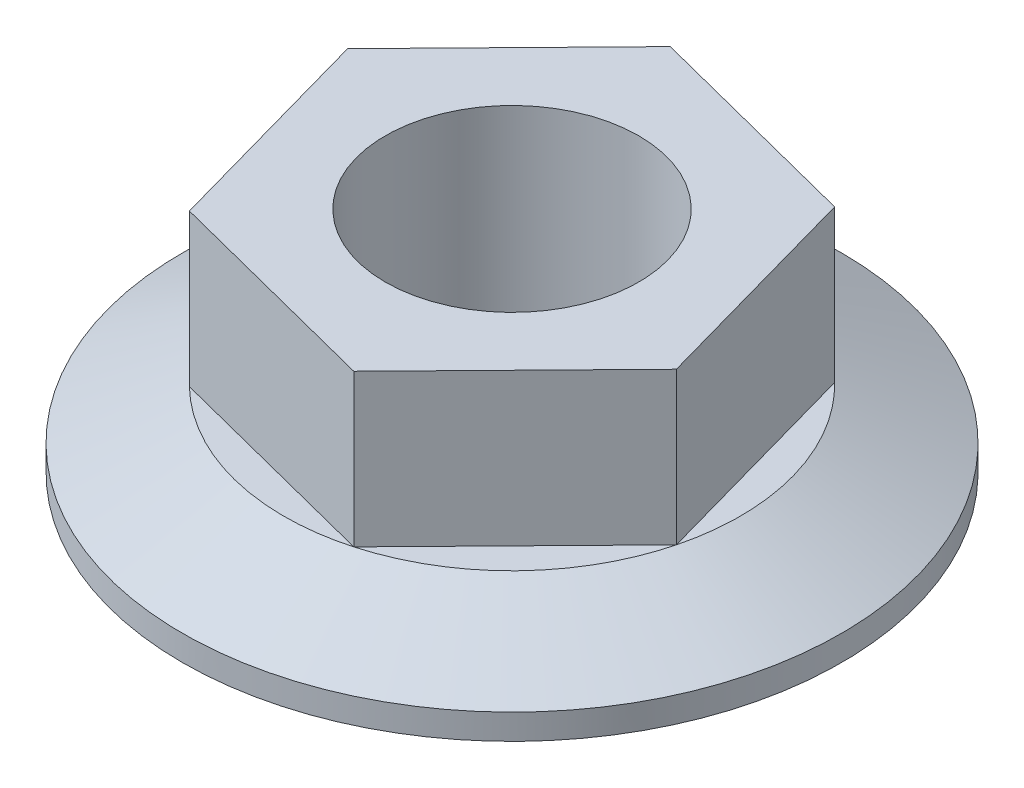
ISO-10303-21;
HEADER;
FILE_DESCRIPTION(('STEP AP214'),'2;1');
FILE_NAME('part.step','',(''),(''),'','','');
FILE_SCHEMA(('AUTOMOTIVE_DESIGN { 1 0 10303 214 1 1 1 1 }'));
ENDSEC;
DATA;
#1=APPLICATION_CONTEXT('core data for automotive mechanical design processes');
#2=APPLICATION_PROTOCOL_DEFINITION('international standard','automotive_design',2000,#1);
#3=PRODUCT_CONTEXT('',#1,'mechanical');
#4=PRODUCT('Part','Part','',(#3));
#5=PRODUCT_RELATED_PRODUCT_CATEGORY('part','',(#4));
#6=PRODUCT_DEFINITION_FORMATION('','',#4);
#7=PRODUCT_DEFINITION_CONTEXT('part definition',#1,'design');
#8=PRODUCT_DEFINITION('design','',#6,#7);
#9=PRODUCT_DEFINITION_SHAPE('','',#8);
#10=(LENGTH_UNIT() NAMED_UNIT(*) SI_UNIT(.MILLI.,.METRE.));
#11=(NAMED_UNIT(*) PLANE_ANGLE_UNIT() SI_UNIT($,.RADIAN.));
#12=(NAMED_UNIT(*) SI_UNIT($,.STERADIAN.) SOLID_ANGLE_UNIT());
#13=UNCERTAINTY_MEASURE_WITH_UNIT(LENGTH_MEASURE(1.E-05),#10,'distance_accuracy_value','');
#14=(GEOMETRIC_REPRESENTATION_CONTEXT(3) GLOBAL_UNCERTAINTY_ASSIGNED_CONTEXT((#13)) GLOBAL_UNIT_ASSIGNED_CONTEXT((#10,
#11,#12)) REPRESENTATION_CONTEXT('',''));
#15=CARTESIAN_POINT('',(0.,0.,0.));
#16=DIRECTION('',(0.,0.,1.));
#17=DIRECTION('',(1.,0.,0.));
#18=AXIS2_PLACEMENT_3D('',#15,#16,#17);
#19=CARTESIAN_POINT('',(0.,1.5,0.));
#20=DIRECTION('',(0.,1.,0.));
#21=DIRECTION('',(0.,0.,1.));
#22=AXIS2_PLACEMENT_3D('',#19,#20,#21);
#23=PLANE('',#22);
#24=CARTESIAN_POINT('',(-3.14677034971334,1.5,3.21680530436099));
#25=CARTESIAN_POINT('',(-2.93612740137397,1.5,3.42286222154896));
#26=CARTESIAN_POINT('',(-2.69997194565525,1.5,3.60002104058776));
#27=CARTESIAN_POINT('',(-2.58257022633489,1.5,3.68809332282499));
#28=CARTESIAN_POINT('',(-2.4587384571172,1.5,3.76889973327667));
#29=CARTESIAN_POINT('',(-2.33582790103386,1.5,3.84910500617602));
#30=CARTESIAN_POINT('',(-2.20697627303336,1.5,3.92163941869568));
#31=CARTESIAN_POINT('',(-2.07908320205732,1.5,3.9936342309657));
#32=CARTESIAN_POINT('',(-1.94576347772724,1.5,4.05758604206279));
#33=CARTESIAN_POINT('',(-1.81343554962159,1.5,4.12106210086509));
#34=CARTESIAN_POINT('',(-1.67621862449045,1.5,4.17615745906585));
#35=CARTESIAN_POINT('',(-1.54002248775998,1.5,4.23084295017093));
#36=CARTESIAN_POINT('',(-1.39949594576583,1.5,4.27684592869383));
#37=CARTESIAN_POINT('',(-1.26001481317743,1.5,4.32250668043339));
#38=CARTESIAN_POINT('',(-1.1167804105469,1.5,4.35922028746182));
#39=CARTESIAN_POINT('',(-0.974611561722385,1.5,4.3956607734873));
#40=CARTESIAN_POINT('',(-0.829282650158769,1.5,4.42292779571922));
#41=CARTESIAN_POINT('',(-0.685034873936298,1.5,4.44999197227462));
#42=CARTESIAN_POINT('',(-0.538233774148871,1.5,4.46769564813512));
#43=CARTESIAN_POINT('',(-0.392524761650793,1.5,4.4852676222617));
#44=CARTESIAN_POINT('',(-0.244880098486916,1.5,4.49333214189259));
#45=CARTESIAN_POINT('',(-0.0983337980726981,1.5,4.50133666769934));
#46=CARTESIAN_POINT('',(0.0495221913514423,1.5,4.49972749758958));
#47=CARTESIAN_POINT('',(0.196278245921577,1.5,4.49813029846792));
#48=CARTESIAN_POINT('',(0.343712419563647,1.5,4.48685432933115));
#49=CARTESIAN_POINT('',(0.49004979633479,1.5,4.47566224473323));
#50=CARTESIAN_POINT('',(0.63643081842759,1.5,4.45476776200012));
#51=CARTESIAN_POINT('',(0.781722878287567,1.5,4.43402871815004));
#52=CARTESIAN_POINT('',(0.926423922820389,1.5,4.40360519520382));
#53=CARTESIAN_POINT('',(1.07031840990569,1.5,4.37335125167627));
#54=CARTESIAN_POINT('',(1.21244993774848,1.5,4.33358571490789));
#55=B_SPLINE_CURVE_WITH_KNOTS('',2,(#24,#25,#26,#27,#28,#29,#30,#31,#32,#33,#34,#35,#36,#37,#38,
#39,#40,#41,#42,#43,#44,#45,#46,#47,#48,#49,#50,#51,#52,#53,#54),.UNSPECIFIED.,.F.,.F.,(3,2,2,2,
2,2,2,2,2,2,2,2,2,2,2,3),(0.,0.125,0.1875,0.25,0.3125,0.375,0.4375,0.5,0.5625,0.625,0.6875,0.75,
0.8125,0.875,0.9375,1.),.UNSPECIFIED.);
#56=CARTESIAN_POINT('',(-3.14677034971334,1.5,3.21680530436099));
#57=VERTEX_POINT('',#56);
#58=CARTESIAN_POINT('',(1.21244944410103,1.5,4.33358395085455));
#59=VERTEX_POINT('',#58);
#60=EDGE_CURVE('E65',#57,#59,#55,.T.);
#61=ORIENTED_EDGE('',*,*,#60,.T.);
#62=DIRECTION('',(-0.96871561943596,0.,-0.248173424565978));
#63=VECTOR('',#62,1.);
#64=CARTESIAN_POINT('',(-0.967160205982432,1.5,3.77519550963444));
#65=LINE('',#64,#63);
#66=EDGE_CURVE('E12',#59,#57,#65,.T.);
#67=ORIENTED_EDGE('',*,*,#66,.T.);
#68=EDGE_LOOP('',(#61,#67));
#69=FACE_BOUND('',#68,.T.);
#70=ADVANCED_FACE('F44',(#69),#23,.T.);
#71=CARTESIAN_POINT('',(1.21244993774848,1.5,4.33358571490789));
#72=CARTESIAN_POINT('',(1.49622193684302,1.5,4.25419202910785));
#73=CARTESIAN_POINT('',(1.76772370250781,1.5,4.13825481472469));
#74=CARTESIAN_POINT('',(1.90269739596185,1.5,4.08061808445978));
#75=CARTESIAN_POINT('',(2.03459368481606,1.5,4.01377983174297));
#76=CARTESIAN_POINT('',(2.1655087667138,1.5,3.94743880422554));
#77=CARTESIAN_POINT('',(2.29275122460852,1.5,3.87211722731326));
#78=CARTESIAN_POINT('',(2.41904709647025,1.5,3.79735598500837));
#79=CARTESIAN_POINT('',(2.54109085166662,1.5,3.71387362245623));
#80=CARTESIAN_POINT('',(2.66222669517993,1.5,3.63101230448085));
#81=CARTESIAN_POINT('',(2.7785491375814,1.5,3.53972664058196));
#82=CARTESIAN_POINT('',(2.89400623046664,1.5,3.44912007182123));
#83=CARTESIAN_POINT('',(3.00410924951721,1.5,3.35042200580243));
#84=CARTESIAN_POINT('',(3.11339318677755,1.5,3.25245817749394));
#85=CARTESIAN_POINT('',(3.21680530444601,1.5,3.14677034962642));
#86=CARTESIAN_POINT('',(3.31944811548519,1.5,3.04186875792201));
#87=CARTESIAN_POINT('',(3.41572650520682,1.5,2.92964373971096));
#88=CARTESIAN_POINT('',(3.51128865774931,1.5,2.81825358933167));
#89=CARTESIAN_POINT('',(3.60002104067895,1.5,2.69997194553367));
#90=CARTESIAN_POINT('',(3.68809332291621,1.5,2.58257022620505));
#91=CARTESIAN_POINT('',(3.76889973336801,1.5,2.45873845697718));
#92=CARTESIAN_POINT('',(3.84910500626744,1.5,2.33582790088381));
#93=CARTESIAN_POINT('',(3.92163941878512,1.5,2.20697627287442));
#94=CARTESIAN_POINT('',(3.99363423105448,1.5,2.07908320188725));
#95=CARTESIAN_POINT('',(4.05758604214822,1.5,1.94576347754909));
#96=CARTESIAN_POINT('',(4.12106210094793,1.5,1.81343554943388));
#97=CARTESIAN_POINT('',(4.17615745914511,1.5,1.67621862429299));
#98=CARTESIAN_POINT('',(4.23084295024639,1.5,1.54002248755345));
#99=CARTESIAN_POINT('',(4.27684592876473,1.5,1.39949594554915));
#100=CARTESIAN_POINT('',(4.32259248864293,1.5,1.25975269249629));
#101=CARTESIAN_POINT('',(4.35922028752217,1.5,1.11678041031134));
#102=B_SPLINE_CURVE_WITH_KNOTS('',2,(#71,#72,#73,#74,#75,#76,#77,#78,#79,#80,#81,#82,#83,#84,
#85,#86,#87,#88,#89,#90,#91,#92,#93,#94,#95,#96,#97,#98,#99,#100,#101),.UNSPECIFIED.,.F.,.F.,(3,
2,2,2,2,2,2,2,2,2,2,2,2,2,2,3),(0.,0.125,0.1875,0.25,0.3125,0.375,0.4375,0.5,0.5625,0.625,
0.6875,0.75,0.8125,0.875,0.9375,1.),.UNSPECIFIED.);
#103=CARTESIAN_POINT('',(4.35922251999599,1.5,1.11678098224459));
#104=VERTEX_POINT('',#103);
#105=EDGE_CURVE('E99',#59,#104,#102,.T.);
#106=ORIENTED_EDGE('',*,*,#105,.T.);
#107=DIRECTION('',(-0.699282299936298,0.,0.714845623191331));
#108=VECTOR('',#107,1.);
#109=CARTESIAN_POINT('',(2.78583511260515,1.5,2.72518306272739));
#110=LINE('',#109,#108);
#111=EDGE_CURVE('E53',#104,#59,#110,.T.);
#112=ORIENTED_EDGE('',*,*,#111,.T.);
#113=EDGE_LOOP('',(#106,#112));
#114=FACE_BOUND('',#113,.T.);
#115=ADVANCED_FACE('F128',(#114),#23,.T.);
#116=CARTESIAN_POINT('',(4.35922028746182,1.5,1.1167804105469));
#117=CARTESIAN_POINT('',(4.43234933819711,1.5,0.831329807583696));
#118=CARTESIAN_POINT('',(4.46769564813002,1.5,0.538233774191154));
#119=CARTESIAN_POINT('',(4.48526762225681,1.5,0.392524761702614));
#120=CARTESIAN_POINT('',(4.49333214188911,1.5,0.244880098550704));
#121=CARTESIAN_POINT('',(4.50133666769727,1.5,0.0983337981482644));
#122=CARTESIAN_POINT('',(4.49972749759051,1.5,-0.0495221912662654));
#123=CARTESIAN_POINT('',(4.49813029847186,1.5,-0.196278245824052));
#124=CARTESIAN_POINT('',(4.48685432933928,1.5,-0.343712419457478));
#125=CARTESIAN_POINT('',(4.47566224474575,1.5,-0.490049796217046));
#126=CARTESIAN_POINT('',(4.45476776201819,1.5,-0.636430818301096));
#127=CARTESIAN_POINT('',(4.43402871817401,1.5,-0.781722878149696));
#128=CARTESIAN_POINT('',(4.40360519523451,1.5,-0.926423922674506));
#129=CARTESIAN_POINT('',(4.37340799990925,1.5,-1.07004850270669));
#130=CARTESIAN_POINT('',(4.33358571495379,1.5,-1.21244993758441));
#131=CARTESIAN_POINT('',(4.29405967717394,1.5,-1.35379201529738));
#132=CARTESIAN_POINT('',(4.24500915534014,1.5,-1.49328405572363));
#133=CARTESIAN_POINT('',(4.1963235316679,1.5,-1.63173838264142));
#134=CARTESIAN_POINT('',(4.13825481482028,1.5,-1.76772370228402));
#135=CARTESIAN_POINT('',(4.08061808456969,1.5,-1.90269739572467));
#136=CARTESIAN_POINT('',(4.0137798318695,1.5,-2.03459368456645));
#137=CARTESIAN_POINT('',(3.94743880436864,1.5,-2.16550876645171));
#138=CARTESIAN_POINT('',(3.87211722747444,1.5,-2.29275122433632));
#139=CARTESIAN_POINT('',(3.79735598518788,1.5,-2.41904709618735));
#140=CARTESIAN_POINT('',(3.71387362265548,1.5,-2.54109085137542));
#141=CARTESIAN_POINT('',(3.63101230470023,1.5,-2.66222669487969));
#142=CARTESIAN_POINT('',(3.53972664082236,1.5,-2.77854913727515));
#143=CARTESIAN_POINT('',(3.4491200720828,1.5,-2.89400623015402));
#144=CARTESIAN_POINT('',(3.3504220060867,1.5,-3.00410924920016));
#145=CARTESIAN_POINT('',(3.2522740788992,1.5,-3.11359855871603));
#146=CARTESIAN_POINT('',(3.14677034995692,1.5,-3.21680530412271));
#147=B_SPLINE_CURVE_WITH_KNOTS('',2,(#116,#117,#118,#119,#120,#121,#122,#123,#124,#125,#126,
#127,#128,#129,#130,#131,#132,#133,#134,#135,#136,#137,#138,#139,#140,#141,#142,#143,#144,#145,
#146),.UNSPECIFIED.,.F.,.F.,(3,2,2,2,2,2,2,2,2,2,2,2,2,2,2,3),(0.,0.125,0.1875,0.25,0.3125,
0.375,0.4375,0.5,0.5625,0.625,0.6875,0.75,0.8125,0.875,0.9375,1.),.UNSPECIFIED.);
#148=CARTESIAN_POINT('',(3.14677198779432,1.5,-3.21680697841206));
#149=VERTEX_POINT('',#148);
#150=EDGE_CURVE('E102',#104,#149,#147,.T.);
#151=ORIENTED_EDGE('',*,*,#150,.T.);
#152=DIRECTION('',(0.269433319499662,0.,0.963019047757308));
#153=VECTOR('',#152,1.);
#154=CARTESIAN_POINT('',(3.75299531858758,1.5,-1.05001244690704));
#155=LINE('',#154,#153);
#156=EDGE_CURVE('E133',#149,#104,#155,.T.);
#157=ORIENTED_EDGE('',*,*,#156,.T.);
#158=EDGE_LOOP('',(#151,#157));
#159=FACE_BOUND('',#158,.T.);
#160=ADVANCED_FACE('F214',(#159),#23,.T.);
#161=CARTESIAN_POINT('',(3.14677034971334,1.5,-3.21680530436099));
#162=CARTESIAN_POINT('',(2.93612740137906,1.5,-3.42286222154397));
#163=CARTESIAN_POINT('',(2.69997194566497,1.5,-3.60002104058047));
#164=CARTESIAN_POINT('',(2.58257022634775,1.5,-3.68809332281592));
#165=CARTESIAN_POINT('',(2.45873845713245,1.5,-3.76889973326672));
#166=CARTESIAN_POINT('',(2.33582790105207,1.5,-3.8491050061648));
#167=CARTESIAN_POINT('',(2.20697627305453,1.5,-3.92163941868377));
#168=CARTESIAN_POINT('',(2.07908320208267,1.5,-3.99363423095239));
#169=CARTESIAN_POINT('',(1.94576347775461,1.5,-4.05758604204967));
#170=CARTESIAN_POINT('',(1.81343554965329,1.5,-4.12106210085104));
#171=CARTESIAN_POINT('',(1.67621862452425,1.5,-4.17615745905228));
#172=CARTESIAN_POINT('',(1.54002248779712,1.5,-4.23084295015734));
#173=CARTESIAN_POINT('',(1.39949594580621,1.5,-4.27684592868062));
#174=CARTESIAN_POINT('',(1.26001481322008,1.5,-4.32250668042086));
#175=CARTESIAN_POINT('',(1.11678041059395,1.5,-4.35922028744976));
#176=CARTESIAN_POINT('',(0.974611561771984,1.5,-4.39566077347619));
#177=CARTESIAN_POINT('',(0.829282650212475,1.5,-4.42292779570915));
#178=CARTESIAN_POINT('',(0.685034873993144,1.5,-4.44999197226576));
#179=CARTESIAN_POINT('',(0.538233774209146,1.5,-4.46769564812786));
#180=CARTESIAN_POINT('',(0.392524761714699,1.5,-4.485267622256));
#181=CARTESIAN_POINT('',(0.244880098553599,1.5,-4.49333214188895));
#182=CARTESIAN_POINT('',(0.0983337981455036,1.5,-4.50133666769757));
#183=CARTESIAN_POINT('',(-0.0495221912785904,1.5,-4.49972749759038));
#184=CARTESIAN_POINT('',(-0.19627824584343,1.5,-4.49813029847132));
#185=CARTESIAN_POINT('',(-0.343712419484948,1.5,-4.48685432933718));
#186=CARTESIAN_POINT('',(-0.490049796253065,1.5,-4.47566224474206));
#187=CARTESIAN_POINT('',(-0.63643081834344,1.5,-4.45476776201215));
#188=CARTESIAN_POINT('',(-0.781722878202335,1.5,-4.43402871816505));
#189=CARTESIAN_POINT('',(-0.926423922731262,1.5,-4.40360519522257));
#190=CARTESIAN_POINT('',(-1.07031840981617,1.5,-4.373351251698));
#191=CARTESIAN_POINT('',(-1.21244993765492,1.5,-4.33358571493406));
#192=B_SPLINE_CURVE_WITH_KNOTS('',2,(#161,#162,#163,#164,#165,#166,#167,#168,#169,#170,#171,
#172,#173,#174,#175,#176,#177,#178,#179,#180,#181,#182,#183,#184,#185,#186,#187,#188,#189,#190,
#191),.UNSPECIFIED.,.F.,.F.,(3,2,2,2,2,2,2,2,2,2,2,2,2,2,2,3),(0.,0.125,0.1875,0.25,0.3125,
0.375,0.4375,0.5,0.5625,0.625,0.6875,0.75,0.8125,0.875,0.9375,1.),.UNSPECIFIED.);
#193=CARTESIAN_POINT('',(-1.21244944410103,1.5,-4.33358395085454));
#194=VERTEX_POINT('',#193);
#195=EDGE_CURVE('E211',#149,#194,#192,.T.);
#196=ORIENTED_EDGE('',*,*,#195,.T.);
#197=DIRECTION('',(0.96871561943596,0.,0.248173424565978));
#198=VECTOR('',#197,1.);
#199=CARTESIAN_POINT('',(0.967160205982431,1.5,-3.77519550963444));
#200=LINE('',#199,#198);
#201=EDGE_CURVE('E423',#194,#149,#200,.T.);
#202=ORIENTED_EDGE('',*,*,#201,.T.);
#203=EDGE_LOOP('',(#196,#202));
#204=FACE_BOUND('',#203,.T.);
#205=ADVANCED_FACE('F291',(#204),#23,.T.);
#206=CARTESIAN_POINT('',(-1.21244993774848,1.5,-4.33358571490789));
#207=CARTESIAN_POINT('',(-1.49622193684344,1.5,-4.25419202910773));
#208=CARTESIAN_POINT('',(-1.76772370250782,1.5,-4.13825481472469));
#209=CARTESIAN_POINT('',(-1.90269739596143,1.5,-4.08061808445993));
#210=CARTESIAN_POINT('',(-2.03459368481606,1.5,-4.01377983174297));
#211=CARTESIAN_POINT('',(-2.16550876671376,1.5,-3.94743880422562));
#212=CARTESIAN_POINT('',(-2.29275122460852,1.5,-3.87211722731326));
#213=CARTESIAN_POINT('',(-2.4190470964708,1.5,-3.79735598500798));
#214=CARTESIAN_POINT('',(-2.54109085166663,1.5,-3.71387362245623));
#215=CARTESIAN_POINT('',(-2.66222669517989,1.5,-3.63101230448089));
#216=CARTESIAN_POINT('',(-2.77854913758141,1.5,-3.53972664058195));
#217=CARTESIAN_POINT('',(-2.89400623046727,1.5,-3.44912007182073));
#218=CARTESIAN_POINT('',(-3.00410924951721,1.5,-3.35042200580242));
#219=CARTESIAN_POINT('',(-3.11339318677746,1.5,-3.25245817749396));
#220=CARTESIAN_POINT('',(-3.21680530444601,1.5,-3.14677034962642));
#221=CARTESIAN_POINT('',(-3.31944811548504,1.5,-3.04186875792223));
#222=CARTESIAN_POINT('',(-3.41572650520682,1.5,-2.92964373971096));
#223=CARTESIAN_POINT('',(-3.51128865774948,1.5,-2.81825358933142));
#224=CARTESIAN_POINT('',(-3.60002104067895,1.5,-2.69997194553366));
#225=CARTESIAN_POINT('',(-3.6880933229159,1.5,-2.58257022620548));
#226=CARTESIAN_POINT('',(-3.76889973336802,1.5,-2.45873845697717));
#227=CARTESIAN_POINT('',(-3.84910500626658,1.5,-2.33582790088517));
#228=CARTESIAN_POINT('',(-3.92163941878513,1.5,-2.20697627287442));
#229=CARTESIAN_POINT('',(-3.99363423105435,1.5,-2.07908320188765));
#230=CARTESIAN_POINT('',(-4.05758604214823,1.5,-1.94576347754908));
#231=CARTESIAN_POINT('',(-4.12106210094796,1.5,-1.81343554943369));
#232=CARTESIAN_POINT('',(-4.17615745914511,1.5,-1.67621862429298));
#233=CARTESIAN_POINT('',(-4.2308429502462,1.5,-1.54002248755403));
#234=CARTESIAN_POINT('',(-4.27684592876474,1.5,-1.39949594554914));
#235=CARTESIAN_POINT('',(-4.32259248864293,1.5,-1.25975269249627));
#236=CARTESIAN_POINT('',(-4.35922028752217,1.5,-1.11678041031133));
#237=B_SPLINE_CURVE_WITH_KNOTS('',2,(#206,#207,#208,#209,#210,#211,#212,#213,#214,#215,#216,
#217,#218,#219,#220,#221,#222,#223,#224,#225,#226,#227,#228,#229,#230,#231,#232,#233,#234,#235,
#236),.UNSPECIFIED.,.F.,.F.,(3,2,2,2,2,2,2,2,2,2,2,2,2,2,2,3),(0.,0.125,0.1875,0.25,0.3125,
0.375,0.4375,0.5,0.5625,0.625,0.6875,0.75,0.8125,0.875,0.9375,1.),.UNSPECIFIED.);
#238=CARTESIAN_POINT('',(-4.35922251999598,1.5,-1.11678098224458));
#239=VERTEX_POINT('',#238);
#240=EDGE_CURVE('E218',#194,#239,#237,.T.);
#241=ORIENTED_EDGE('',*,*,#240,.T.);
#242=DIRECTION('',(0.699282299936298,0.,-0.714845623191331));
#243=VECTOR('',#242,1.);
#244=CARTESIAN_POINT('',(-2.78583511260515,1.5,-2.7251830627274));
#245=LINE('',#244,#243);
#246=EDGE_CURVE('E232',#239,#194,#245,.T.);
#247=ORIENTED_EDGE('',*,*,#246,.T.);
#248=EDGE_LOOP('',(#241,#247));
#249=FACE_BOUND('',#248,.T.);
#250=ADVANCED_FACE('F286',(#249),#23,.T.);
#251=CARTESIAN_POINT('',(-4.35922028746182,1.5,-1.11678041054689));
#252=CARTESIAN_POINT('',(-4.43234933820224,1.5,-0.831329807563667));
#253=CARTESIAN_POINT('',(-4.46769564813512,1.5,-0.538233774148863));
#254=CARTESIAN_POINT('',(-4.4852676222617,1.5,-0.392524761650791));
#255=CARTESIAN_POINT('',(-4.49333214189259,1.5,-0.244880098486908));
#256=CARTESIAN_POINT('',(-4.50133666769934,1.5,-0.0983337980727092));
#257=CARTESIAN_POINT('',(-4.49972749758958,1.5,0.0495221913514494));
#258=CARTESIAN_POINT('',(-4.49813029846792,1.5,0.196278245921584));
#259=CARTESIAN_POINT('',(-4.48685432933115,1.5,0.343712419563654));
#260=CARTESIAN_POINT('',(-4.47566224473337,1.5,0.490049796332997));
#261=CARTESIAN_POINT('',(-4.45476776200012,1.5,0.636430818427593));
#262=CARTESIAN_POINT('',(-4.4340287181504,1.5,0.781722878285904));
#263=CARTESIAN_POINT('',(-4.40360519520382,1.5,0.926423922820388));
#264=CARTESIAN_POINT('',(-4.37340799987167,1.5,1.07004850286154));
#265=CARTESIAN_POINT('',(-4.33358571490789,1.5,1.21244993774848));
#266=CARTESIAN_POINT('',(-4.29405967711975,1.5,1.35379201547067));
#267=CARTESIAN_POINT('',(-4.24500915527653,1.5,1.49328405590444));
#268=CARTESIAN_POINT('',(-4.19632353159432,1.5,1.63173838283148));
#269=CARTESIAN_POINT('',(-4.13825481473663,1.5,1.76772370247986));
#270=CARTESIAN_POINT('',(-4.08061808447537,1.5,1.9026973959278));
#271=CARTESIAN_POINT('',(-4.01377983176358,1.5,2.03459368477539));
#272=CARTESIAN_POINT('',(-3.94743880425134,1.5,2.16550876666618));
#273=CARTESIAN_POINT('',(-3.87211722734423,1.5,2.29275122455622));
#274=CARTESIAN_POINT('',(-3.79735598504567,1.5,2.41904709641129));
#275=CARTESIAN_POINT('',(-3.71387362249914,1.5,2.54109085160391));
#276=CARTESIAN_POINT('',(-3.63101230453054,1.5,2.66222669511173));
#277=CARTESIAN_POINT('',(-3.53972664063826,1.5,2.77854913750968));
#278=CARTESIAN_POINT('',(-3.4491200718842,1.5,2.89400623039128));
#279=CARTESIAN_POINT('',(-3.35042200587345,1.5,3.004109249438));
#280=CARTESIAN_POINT('',(-3.25227407867076,1.5,3.11359855895513));
#281=CARTESIAN_POINT('',(-3.14677034971334,1.5,3.21680530436099));
#282=B_SPLINE_CURVE_WITH_KNOTS('',2,(#251,#252,#253,#254,#255,#256,#257,#258,#259,#260,#261,
#262,#263,#264,#265,#266,#267,#268,#269,#270,#271,#272,#273,#274,#275,#276,#277,#278,#279,#280,
#281),.UNSPECIFIED.,.F.,.F.,(3,2,2,2,2,2,2,2,2,2,2,2,2,2,2,3),(0.,0.125,0.1875,0.25,0.3125,
0.375,0.4375,0.5,0.5625,0.625,0.6875,0.75,0.8125,0.875,0.9375,1.),.UNSPECIFIED.);
#283=EDGE_CURVE('E135',#239,#57,#282,.T.);
#284=ORIENTED_EDGE('',*,*,#283,.T.);
#285=DIRECTION('',(-0.269433319499662,0.,-0.963019047757308));
#286=VECTOR('',#285,1.);
#287=CARTESIAN_POINT('',(-3.75299531858758,1.5,1.05001244690704));
#288=LINE('',#287,#286);
#289=EDGE_CURVE('E224',#57,#239,#288,.T.);
#290=ORIENTED_EDGE('',*,*,#289,.T.);
#291=EDGE_LOOP('',(#284,#290));
#292=FACE_BOUND('',#291,.T.);
#293=ADVANCED_FACE('F153',(#292),#23,.T.);
#294=CARTESIAN_POINT('',(-0.967160205982432,4.5,3.77519550963444));
#295=DIRECTION('',(0.248173424565978,0.,-0.96871561943596));
#296=DIRECTION('',(-0.96871561943596,0.,-0.248173424565978));
#297=AXIS2_PLACEMENT_3D('',#294,#295,#296);
#298=PLANE('',#297);
#299=ORIENTED_EDGE('',*,*,#66,.F.);
#300=DIRECTION('',(0.,-1.,0.));
#301=VECTOR('',#300,1.);
#302=CARTESIAN_POINT('',(1.21244993774848,4.5,4.33358571490789));
#303=LINE('',#302,#301);
#304=CARTESIAN_POINT('',(1.21244993774848,4.5,4.33358571490789));
#305=VERTEX_POINT('',#304);
#306=EDGE_CURVE('E118',#305,#59,#303,.T.);
#307=ORIENTED_EDGE('',*,*,#306,.F.);
#308=DIRECTION('',(0.96871561943596,0.,0.248173424565978));
#309=VECTOR('',#308,1.);
#310=CARTESIAN_POINT('',(-0.967160205982432,4.5,3.77519550963444));
#311=LINE('',#310,#309);
#312=CARTESIAN_POINT('',(-3.14677034971334,4.5,3.21680530436099));
#313=VERTEX_POINT('',#312);
#314=EDGE_CURVE('E246',#313,#305,#311,.T.);
#315=ORIENTED_EDGE('',*,*,#314,.F.);
#316=DIRECTION('',(0.,-1.,0.));
#317=VECTOR('',#316,1.);
#318=CARTESIAN_POINT('',(-3.14677034971334,4.5,3.21680530436099));
#319=LINE('',#318,#317);
#320=EDGE_CURVE('E119',#313,#57,#319,.T.);
#321=ORIENTED_EDGE('',*,*,#320,.T.);
#322=EDGE_LOOP('',(#299,#307,#315,#321));
#323=FACE_BOUND('',#322,.T.);
#324=ADVANCED_FACE('F120',(#323),#298,.F.);
#325=CARTESIAN_POINT('',(2.78583511260515,4.5,2.72518306272739));
#326=DIRECTION('',(-0.714845623191331,0.,-0.699282299936297));
#327=DIRECTION('',(-0.699282299936298,0.,0.714845623191331));
#328=AXIS2_PLACEMENT_3D('',#325,#326,#327);
#329=PLANE('',#328);
#330=ORIENTED_EDGE('',*,*,#111,.F.);
#331=DIRECTION('',(0.,-1.,0.));
#332=VECTOR('',#331,1.);
#333=CARTESIAN_POINT('',(4.35922028746182,4.5,1.1167804105469));
#334=LINE('',#333,#332);
#335=CARTESIAN_POINT('',(4.35922028746182,4.5,1.1167804105469));
#336=VERTEX_POINT('',#335);
#337=EDGE_CURVE('E129',#336,#104,#334,.T.);
#338=ORIENTED_EDGE('',*,*,#337,.F.);
#339=DIRECTION('',(0.699282299936297,0.,-0.714845623191331));
#340=VECTOR('',#339,1.);
#341=CARTESIAN_POINT('',(2.78583511260515,4.5,2.72518306272739));
#342=LINE('',#341,#340);
#343=EDGE_CURVE('E130',#305,#336,#342,.T.);
#344=ORIENTED_EDGE('',*,*,#343,.F.);
#345=ORIENTED_EDGE('',*,*,#306,.T.);
#346=EDGE_LOOP('',(#330,#338,#344,#345));
#347=FACE_BOUND('',#346,.T.);
#348=ADVANCED_FACE('F121',(#347),#329,.F.);
#349=CARTESIAN_POINT('',(3.75299531858758,4.5,-1.05001244690704));
#350=DIRECTION('',(-0.963019047757308,0.,0.269433319499662));
#351=DIRECTION('',(0.269433319499662,0.,0.963019047757308));
#352=AXIS2_PLACEMENT_3D('',#349,#350,#351);
#353=PLANE('',#352);
#354=ORIENTED_EDGE('',*,*,#156,.F.);
#355=DIRECTION('',(0.,-1.,0.));
#356=VECTOR('',#355,1.);
#357=CARTESIAN_POINT('',(3.14677034971334,4.5,-3.21680530436099));
#358=LINE('',#357,#356);
#359=CARTESIAN_POINT('',(3.14677034971334,4.5,-3.21680530436099));
#360=VERTEX_POINT('',#359);
#361=EDGE_CURVE('E192',#360,#149,#358,.T.);
#362=ORIENTED_EDGE('',*,*,#361,.F.);
#363=DIRECTION('',(-0.269433319499662,0.,-0.963019047757309));
#364=VECTOR('',#363,1.);
#365=CARTESIAN_POINT('',(3.75299531858758,4.5,-1.05001244690704));
#366=LINE('',#365,#364);
#367=EDGE_CURVE('E243',#336,#360,#366,.T.);
#368=ORIENTED_EDGE('',*,*,#367,.F.);
#369=ORIENTED_EDGE('',*,*,#337,.T.);
#370=EDGE_LOOP('',(#354,#362,#368,#369));
#371=FACE_BOUND('',#370,.T.);
#372=ADVANCED_FACE('F283',(#371),#353,.F.);
#373=CARTESIAN_POINT('',(0.967160205982431,4.5,-3.77519550963444));
#374=DIRECTION('',(-0.248173424565978,0.,0.96871561943596));
#375=DIRECTION('',(0.96871561943596,0.,0.248173424565978));
#376=AXIS2_PLACEMENT_3D('',#373,#374,#375);
#377=PLANE('',#376);
#378=ORIENTED_EDGE('',*,*,#201,.F.);
#379=DIRECTION('',(0.,-1.,0.));
#380=VECTOR('',#379,1.);
#381=CARTESIAN_POINT('',(-1.21244993774848,4.5,-4.33358571490789));
#382=LINE('',#381,#380);
#383=CARTESIAN_POINT('',(-1.21244993774848,4.5,-4.33358571490789));
#384=VERTEX_POINT('',#383);
#385=EDGE_CURVE('E197',#384,#194,#382,.T.);
#386=ORIENTED_EDGE('',*,*,#385,.F.);
#387=DIRECTION('',(-0.96871561943596,0.,-0.248173424565978));
#388=VECTOR('',#387,1.);
#389=CARTESIAN_POINT('',(0.967160205982431,4.5,-3.77519550963444));
#390=LINE('',#389,#388);
#391=EDGE_CURVE('E241',#360,#384,#390,.T.);
#392=ORIENTED_EDGE('',*,*,#391,.F.);
#393=ORIENTED_EDGE('',*,*,#361,.T.);
#394=EDGE_LOOP('',(#378,#386,#392,#393));
#395=FACE_BOUND('',#394,.T.);
#396=ADVANCED_FACE('F280',(#395),#377,.F.);
#397=CARTESIAN_POINT('',(-2.78583511260515,4.5,-2.7251830627274));
#398=DIRECTION('',(0.714845623191331,0.,0.699282299936298));
#399=DIRECTION('',(0.699282299936298,0.,-0.714845623191331));
#400=AXIS2_PLACEMENT_3D('',#397,#398,#399);
#401=PLANE('',#400);
#402=ORIENTED_EDGE('',*,*,#246,.F.);
#403=DIRECTION('',(0.,-1.,0.));
#404=VECTOR('',#403,1.);
#405=CARTESIAN_POINT('',(-4.35922028746182,4.5,-1.1167804105469));
#406=LINE('',#405,#404);
#407=CARTESIAN_POINT('',(-4.35922028746182,4.5,-1.1167804105469));
#408=VERTEX_POINT('',#407);
#409=EDGE_CURVE('E207',#408,#239,#406,.T.);
#410=ORIENTED_EDGE('',*,*,#409,.F.);
#411=DIRECTION('',(-0.699282299936298,0.,0.714845623191331));
#412=VECTOR('',#411,1.);
#413=CARTESIAN_POINT('',(-2.78583511260515,4.5,-2.7251830627274));
#414=LINE('',#413,#412);
#415=EDGE_CURVE('E237',#384,#408,#414,.T.);
#416=ORIENTED_EDGE('',*,*,#415,.F.);
#417=ORIENTED_EDGE('',*,*,#385,.T.);
#418=EDGE_LOOP('',(#402,#410,#416,#417));
#419=FACE_BOUND('',#418,.T.);
#420=ADVANCED_FACE('F274',(#419),#401,.F.);
#421=CARTESIAN_POINT('',(0.,4.5,0.));
#422=DIRECTION('',(0.,-1.,0.));
#423=DIRECTION('',(0.,0.,-1.));
#424=AXIS2_PLACEMENT_3D('',#421,#422,#423);
#425=CYLINDRICAL_SURFACE('',#424,2.5);
#426=CARTESIAN_POINT('',(0.,4.5,0.));
#427=DIRECTION('',(0.,1.,0.));
#428=DIRECTION('',(0.,0.,1.));
#429=AXIS2_PLACEMENT_3D('',#426,#427,#428);
#430=CIRCLE('',#429,2.5);
#431=CARTESIAN_POINT('',(0.,4.5,2.5));
#432=VERTEX_POINT('',#431);
#433=EDGE_CURVE('E247',#432,#432,#430,.T.);
#434=ORIENTED_EDGE('',*,*,#433,.T.);
#435=EDGE_LOOP('',(#434));
#436=FACE_BOUND('',#435,.T.);
#437=CARTESIAN_POINT('',(0.,0.,0.));
#438=DIRECTION('',(0.,1.,0.));
#439=DIRECTION('',(0.,0.,1.));
#440=AXIS2_PLACEMENT_3D('',#437,#438,#439);
#441=CIRCLE('',#440,2.5);
#442=CARTESIAN_POINT('',(0.,0.,2.5));
#443=VERTEX_POINT('',#442);
#444=EDGE_CURVE('E47',#443,#443,#441,.T.);
#445=ORIENTED_EDGE('',*,*,#444,.F.);
#446=EDGE_LOOP('',(#445));
#447=FACE_BOUND('',#446,.T.);
#448=ADVANCED_FACE('F154',(#436,#447),#425,.F.);
#449=CARTESIAN_POINT('',(-3.75299531858758,4.5,1.05001244690705));
#450=DIRECTION('',(0.963019047757308,0.,-0.269433319499662));
#451=DIRECTION('',(-0.269433319499662,0.,-0.963019047757308));
#452=AXIS2_PLACEMENT_3D('',#449,#450,#451);
#453=PLANE('',#452);
#454=ORIENTED_EDGE('',*,*,#289,.F.);
#455=ORIENTED_EDGE('',*,*,#320,.F.);
#456=DIRECTION('',(0.269433319499662,0.,0.963019047757309));
#457=VECTOR('',#456,1.);
#458=CARTESIAN_POINT('',(-3.75299531858758,4.5,1.05001244690705));
#459=LINE('',#458,#457);
#460=EDGE_CURVE('E72',#408,#313,#459,.T.);
#461=ORIENTED_EDGE('',*,*,#460,.F.);
#462=ORIENTED_EDGE('',*,*,#409,.T.);
#463=EDGE_LOOP('',(#454,#455,#461,#462));
#464=FACE_BOUND('',#463,.T.);
#465=ADVANCED_FACE('F266',(#464),#453,.F.);
#466=CARTESIAN_POINT('',(0.,4.5,0.));
#467=DIRECTION('',(0.,1.,0.));
#468=DIRECTION('',(0.,0.,1.));
#469=AXIS2_PLACEMENT_3D('',#466,#467,#468);
#470=PLANE('',#469);
#471=ORIENTED_EDGE('',*,*,#433,.F.);
#472=EDGE_LOOP('',(#471));
#473=FACE_BOUND('',#472,.T.);
#474=ORIENTED_EDGE('',*,*,#314,.T.);
#475=ORIENTED_EDGE('',*,*,#343,.T.);
#476=ORIENTED_EDGE('',*,*,#367,.T.);
#477=ORIENTED_EDGE('',*,*,#391,.T.);
#478=ORIENTED_EDGE('',*,*,#415,.T.);
#479=ORIENTED_EDGE('',*,*,#460,.T.);
#480=EDGE_LOOP('',(#474,#475,#476,#477,#478,#479));
#481=FACE_BOUND('',#480,.T.);
#482=ADVANCED_FACE('F261',(#473,#481),#470,.T.);
#483=CARTESIAN_POINT('',(0.,1.5,0.));
#484=DIRECTION('',(0.,-1.,0.));
#485=DIRECTION('',(0.,0.,-1.));
#486=AXIS2_PLACEMENT_3D('',#483,#484,#485);
#487=CONICAL_SURFACE('',#486,4.5,1.10714871779409);
#488=CARTESIAN_POINT('',(0.,0.5,0.));
#489=DIRECTION('',(0.,-1.,0.));
#490=DIRECTION('',(0.,0.,-1.));
#491=AXIS2_PLACEMENT_3D('',#488,#489,#490);
#492=CIRCLE('',#491,6.5);
#493=CARTESIAN_POINT('',(0.,0.5,-6.5));
#494=VERTEX_POINT('',#493);
#495=EDGE_CURVE('E145',#494,#494,#492,.F.);
#496=ORIENTED_EDGE('',*,*,#495,.T.);
#497=EDGE_LOOP('',(#496));
#498=FACE_BOUND('',#497,.T.);
#499=ORIENTED_EDGE('',*,*,#105,.F.);
#500=ORIENTED_EDGE('',*,*,#60,.F.);
#501=ORIENTED_EDGE('',*,*,#283,.F.);
#502=ORIENTED_EDGE('',*,*,#240,.F.);
#503=ORIENTED_EDGE('',*,*,#195,.F.);
#504=ORIENTED_EDGE('',*,*,#150,.F.);
#505=EDGE_LOOP('',(#499,#500,#501,#502,#503,#504));
#506=FACE_BOUND('',#505,.T.);
#507=ADVANCED_FACE('F101',(#498,#506),#487,.T.);
#508=CARTESIAN_POINT('',(0.,0.,0.));
#509=DIRECTION('',(0.,1.,0.));
#510=DIRECTION('',(0.,0.,1.));
#511=AXIS2_PLACEMENT_3D('',#508,#509,#510);
#512=PLANE('',#511);
#513=ORIENTED_EDGE('',*,*,#444,.T.);
#514=EDGE_LOOP('',(#513));
#515=FACE_BOUND('',#514,.T.);
#516=CARTESIAN_POINT('',(0.,0.,0.));
#517=DIRECTION('',(0.,1.,0.));
#518=DIRECTION('',(0.,0.,1.));
#519=AXIS2_PLACEMENT_3D('',#516,#517,#518);
#520=CIRCLE('',#519,6.5);
#521=CARTESIAN_POINT('',(0.,0.,6.5));
#522=VERTEX_POINT('',#521);
#523=EDGE_CURVE('E111',#522,#522,#520,.T.);
#524=ORIENTED_EDGE('',*,*,#523,.F.);
#525=EDGE_LOOP('',(#524));
#526=FACE_BOUND('',#525,.T.);
#527=ADVANCED_FACE('F155',(#515,#526),#512,.F.);
#528=CARTESIAN_POINT('',(0.,0.5,0.));
#529=DIRECTION('',(0.,-1.,0.));
#530=DIRECTION('',(0.,0.,-1.));
#531=AXIS2_PLACEMENT_3D('',#528,#529,#530);
#532=CYLINDRICAL_SURFACE('',#531,6.5);
#533=ORIENTED_EDGE('',*,*,#495,.F.);
#534=EDGE_LOOP('',(#533));
#535=FACE_BOUND('',#534,.T.);
#536=ORIENTED_EDGE('',*,*,#523,.T.);
#537=EDGE_LOOP('',(#536));
#538=FACE_BOUND('',#537,.T.);
#539=ADVANCED_FACE('F50',(#535,#538),#532,.T.);
#540=CLOSED_SHELL('',(#70,#115,#160,#205,#250,#293,#324,#348,#372,#396,#420,#448,#465,#482,#507,
#527,#539));
#541=MANIFOLD_SOLID_BREP('B2',#540);
#542=ADVANCED_BREP_SHAPE_REPRESENTATION('',(#18,#541),#14);
#543=SHAPE_DEFINITION_REPRESENTATION(#9,#542);
ENDSEC;
END-ISO-10303-21;
